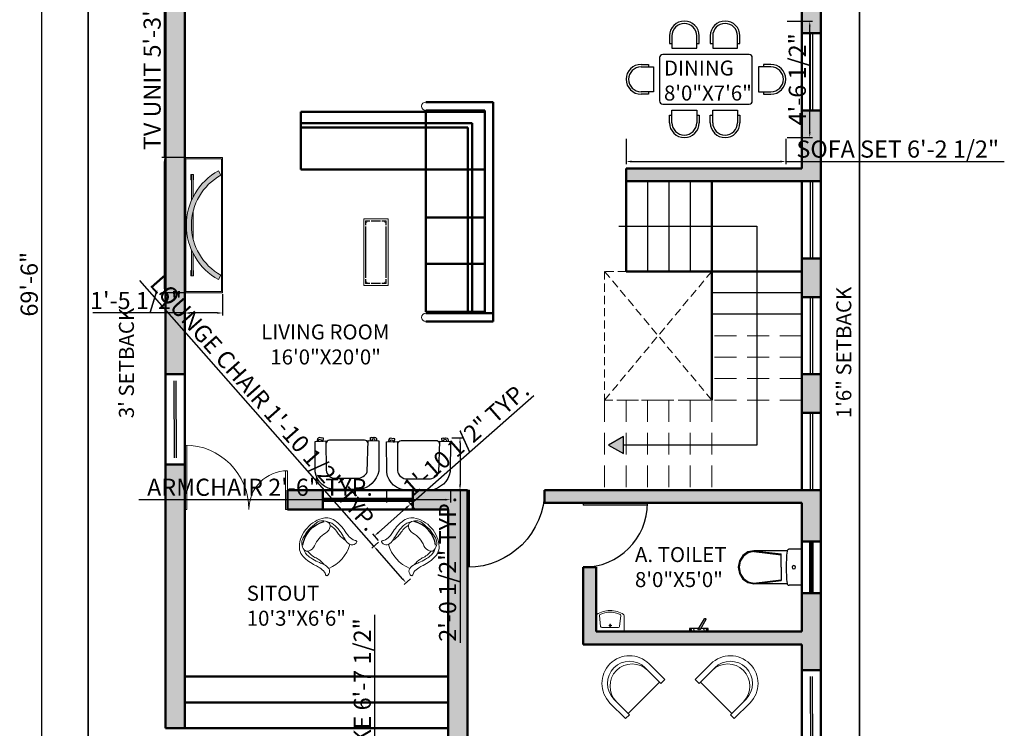
# Model space of a CAD drawing. Units: inches. Extents: x 1986 to 21484, y -1816 to 2016.
# Tile 5 of 85: x 2010 to 2470, y 1277 to 1607. Entities that reach past the tile are written whole.
import ezdxf

# ---------------------------------------------------------------- set-up
doc = ezdxf.new("R2010")
doc.units = ezdxf.units.IN
doc.linetypes.add('DASHED', pattern=[19.05, 12.7, -6.35])
for name, color, linetype in [('2D', 7, 'Continuous'), ('IFF-FURN-DETAIL', 250, 'Continuous'), ('NOI THAT', 42, 'Continuous'), ('SANTEH', 7, 'Continuous')]:
    doc.layers.add(name, color=color, linetype=linetype)
for name, color, linetype, lineweight in [('A-ANNO-DIMS', 2, 'Continuous', 18), ('A-ANNO-TEXT', 7, 'Continuous', 18), ('A-AREA-IDEN', 3, 'Continuous', 18), ('A-DOOR', 3, 'Continuous', 25), ('A-FLOR-FIXT', 8, 'Continuous', 18), ('A-FLOR-STRS', 7, 'Continuous', 25), ('A-FLOR-STRS-OVHD', 8, 'DASHED', 18), ('A-FURN', 8, 'Continuous', 18), ('A-GLAZ', 4, 'Continuous', 25), ('A-WALL', 7, 'Continuous', 50), ('A-WALL-PATT', 8, 'Continuous', 13), ('aparador', 36, 'Continuous', 9), ('C-PROP', 7, 'Continuous', 35), ('moveis', 254, 'Continuous', 5)]:
    doc.layers.add(name, color=color, linetype=linetype, lineweight=lineweight)
doc.styles.get("Standard").update_dxf_attribs({"font": 'arial.ttf'})
doc.dimstyles.new('ISO-25', dxfattribs={"dimtxt": 8, "dimasz": 2.5, "dimexe": 1.25, "dimexo": 0.625, "dimtad": 1, "dimdec": 1, "dimlunit": 3, "dimtxsty": 'Standard', "dimcen": 2.5, "dimadec": 0, "dimazin": 0, "dimtfac": 1, "dimtdec": 1, "dimtmove": 0, "dimatfit": 3, "dimfxl": 1, "dimarcsym": 0})

# ---------------------------------------------------------------- blocks, each defined once
blk = doc.blocks.new('*D2')
at = {"layer": 'A-ANNO-DIMS', "color": 0, "lineweight": -2, "transparency": 16777216}
for p, q in [((2041.69, 1900.75), (2019.21, 1900.75)), ((2020.46, 1898.25), (2020.46, 1069.25)), ((2041.69, 1066.75), (2019.21, 1066.75))]:
    blk.add_line(p, q, dxfattribs=at)
at = {"layer": 'A-ANNO-DIMS', "color": 0, "transparency": 16777216}
for points in [[(2020.05, 1898.25), (2020.88, 1898.25), (2020.46, 1900.75)], [(2020.05, 1069.25), (2020.88, 1069.25), (2020.46, 1066.75)]]:
    blk.add_solid(points, dxfattribs=at)
at = {"layer": 'Defpoints', "color": 0, "transparency": 16777216}
for p in [(2042.31, 1900.75), (2020.46, 1066.75), (2042.31, 1066.75)]:
    blk.add_point(p, dxfattribs=at)
at = {"layer": 'A-ANNO-DIMS', "color": 0, "transparency": 16777216, "insert": (2015.75, 1483.75), "char_height": 8, "attachment_point": 5, "rotation": 90}
blk.add_mtext('69\'-6"', dxfattribs=at)
blk = doc.blocks.new('MD')
for p, q in [((1902.58, 1512.86), (1902.58, 1482.86)), ((1903.58, 1512.86), (1903.58, 1482.86)), ((1949.58, 1482.86), (1949.58, 1500.86)), ((1950.58, 1482.86), (1950.58, 1500.86)), ((1902.58, 1482.86), (1903.58, 1482.86)), ((1949.58, 1482.86), (1950.58, 1482.86))]:
    blk.add_line(p, q)
for centre, radius, start, end in [((1902.58, 1482.86), 30, 0, 90), ((1950.58, 1482.86), 18, 90, 180)]:
    blk.add_arc(centre, radius, start, end)
blk = doc.blocks.new('D2')
for p, q in [((1722.5, 1505.46), (1722.5, 1475.46)), ((1723.5, 1505.46), (1723.5, 1475.46)), ((1722.5, 1475.46), (1723.5, 1475.46))]:
    blk.add_line(p, q)
blk.add_arc((1722.5, 1475.46), 30, 0, 90)
blk = doc.blocks.new('D1')
for p, q in [((1805.96, 1500.36), (1805.96, 1464.36)), ((1806.96, 1500.36), (1806.96, 1464.36)), ((1805.96, 1464.36), (1806.96, 1464.36))]:
    blk.add_line(p, q)
blk.add_arc((1805.96, 1464.36), 36, 0, 90)
blk = doc.blocks.new('WC 2 Symb_109')
at = {"layer": 'SANTEH'}
for p, q in [((0, 0), (0, 380)), ((0, 380), (132, 380)), ((154, 365), (507, 365)), ((506, 365), (216, 331)), ((506, 356), (216, 322)), ((216, 190), (216, 331)), ((216, 190), (216, 49)), ((154, 15), (507, 15)), ((506, 24), (216, 58)), ((506, 15), (216, 49)), ((0, 0), (132, 0))]:
    blk.add_line(p, q, dxfattribs=at)
for points in [[(155, 360), (154, 364), (152, 368), (150, 371), (147, 374), (144, 377), (140, 379), (137, 380), (132, 380)], [(155, 20), (159, 62), (161, 105), (163, 147), (164, 190), (163, 233), (161, 275), (159, 318), (155, 360)], [(506, 24), (565, 37), (616, 73), (649, 126), (661, 190), (649, 254), (616, 307), (565, 343), (506, 356)], [(507, 15), (569, 28), (622, 66), (658, 123), (670, 190), (658, 257), (622, 314), (569, 352), (507, 365)], [(132, 0), (136, 0), (140, 1), (144, 3), (147, 6), (150, 9), (152, 12), (154, 16), (155, 20)]]:
    blk.add_lwpolyline(points, dxfattribs=at)
blk.add_lwpolyline([(84, 208), (70, 203), (65, 190), (70, 177), (84, 172), (97, 177), (102, 190), (97, 203)], close=True, dxfattribs=at)
blk = doc.blocks.new('Faucet - kit sink top')
at = {"layer": 'SANTEH'}
for p, q in [((-5.5, -0.75), (-5.5, -1.25)), ((-4.94278, -0.75), (-5.5, -0.75)), ((-5.5, -1.25), (-4.94278, -1.25)), ((-0.14775, -1.7441), (3.56698, -8.1782)), ((4.43301, -7.6782), (0.71828, -1.2441)), ((4.94278, -0.75), (5.5, -0.75)), ((5.5, -1.25), (4.94278, -1.25)), ((5.5, -0.75), (5.5, -1.25))]:
    blk.add_line(p, q, dxfattribs=at)
blk.add_lwpolyline([(-0.00587, -2), (-6, -2), (-6, 0), (6, 0), (6, -2), (1.15195, -2)], dxfattribs=at)
for centre, radius in [((-4, -1), 1), ((4, -1), 1), ((0, -1), 0.75)]:
    blk.add_circle(centre, radius, dxfattribs=at)
blk.add_arc((4, -7.9282), 0.5, 210, 30, dxfattribs=at)
blk = doc.blocks.new('A$C2EBB240D')
for p, q in [((0, 356), (0, 87)), ((480, 376), (20, 376)), ((500, 356), (500, 87)), ((61, 90), (82, 282)), ((250, 300), (102, 300)), ((250, 300), (398, 300)), ((439, 90), (418, 282))]:
    blk.add_line(p, q)
for points in [[(275, 266), (219, 266)], [(247, 238), (247, 289)]]:
    blk.add_lwpolyline(points)
for centre, radius, start, end in [((20, 356), 20, 90, 180), ((480, 356), 20, 0, 90), ((102, 280), 20, 90, 173.6428), ((247, 266), 16.7, 90, 270), ((247, 266), 10, 90, 270), ((247, 266), 16.7, 270, 90), ((247, 266), 10, 270, 90), ((398, 280), 20, 6.3572, 90), ((20, 87), 20, 180, 237.6892), ((250, 450), 450, 237.6892, 270), ((81, 88), 20, 173.6428, 244.9796), ((250, 450), 420, 244.9796, 270), ((250, 450), 450, 270, 302.3108), ((250, 450), 420, 270, 295.0204), ((419, 88), 20, 295.0204, 6.3572), ((480, 87), 20, 302.3108, 0)]:
    blk.add_arc(centre, radius, start, end)
blk = doc.blocks.new('A$C3F0C2877')
at = {"layer": 'NOI THAT'}
for p, q in [((700, 1640), (700, 1520)), ((740, 1640), (740, 1440)), ((1140, 1440), (1140, 1640)), ((1180, 1520), (1180, 1640)), ((1358, 1640), (1358, 1520)), ((1398, 1640), (1398, 1440)), ((1798, 1440), (1798, 1640)), ((1838, 1520), (1838, 1640)), ((700, 1520), (740, 1520)), ((740, 1440), (1140, 1440)), ((1140, 1520), (1180, 1520)), ((1358, 1520), (1398, 1520)), ((1398, 1440), (1798, 1440)), ((1798, 1520), (1838, 1520)), ((540, 1290), (540, 590)), ((1988, 1340), (590, 1340)), ((2038, 590), (2038, 1290)), ((240, 1180), (360, 1180)), ((240, 1140), (440, 1140)), ((360, 1180), (360, 1140)), ((440, 1140), (440, 740)), ((2139, 1140), (2139, 740)), ((2339, 1140), (2139, 1140)), ((2339, 1180), (2219, 1180)), ((2219, 1180), (2219, 1140)), ((440, 740), (240, 740)), ((360, 700), (240, 700)), ((360, 740), (360, 700)), ((2139, 740), (2339, 740)), ((2219, 740), (2219, 700)), ((2219, 700), (2339, 700)), ((590, 540), (1988, 540)), ((700, 360), (740, 360)), ((700, 240), (700, 360)), ((740, 440), (1140, 440)), ((740, 240), (740, 440)), ((1140, 440), (1140, 240)), ((1140, 360), (1180, 360)), ((1180, 360), (1180, 240)), ((1358, 360), (1398, 360)), ((1358, 240), (1358, 360)), ((1398, 440), (1798, 440)), ((1398, 240), (1398, 440)), ((1798, 440), (1798, 240)), ((1798, 360), (1838, 360)), ((1838, 360), (1838, 240))]:
    blk.add_line(p, q, dxfattribs=at)
for centre, radius, start, end in [((940, 1640), 240, 0, 180), ((940, 1640), 200, 0, 180), ((1598, 1640), 240, 0, 180), ((1598, 1640), 200, 0, 180), ((590, 1290), 50, 90, 180), ((1988, 1290), 50, 0, 90), ((240, 940), 240, 90, 270), ((240, 940), 200, 90, 270), ((2339, 940), 240, 270, 90), ((2339, 940), 200, 270, 90), ((590, 590), 50, 180, 270), ((1988, 590), 50, 270, 0), ((940, 240), 240, 180, 0), ((940, 240), 200, 180, 0), ((1598, 240), 240, 180, 0), ((1598, 240), 200, 180, 0)]:
    blk.add_arc(centre, radius, start, end, dxfattribs=at)
blk = doc.blocks.new('ILNG95')
for points in [[(120, 308, -0.32971), (51, 384, -0.036099), (50, 422, -0.497733), (75, 439, -0.070621), (96, 429, 0.101868), (133, 414, 0.091794), (259, 412, 0.024114), (351, 433, -0.090294), (638, 458, -0.132412), (775, 407, -0.068618), (816, 368, -0.184346), (943, 0, 1.803905)], [(120, 308, 0.138132), (244, 313, 0.001085), (325, 339, -0.034227), (462, 375, -0.033255), (567, 387, -0.137428), (727, 350, -4.561553)], [(120, 308, 0.138132), (244, 313, 0.001085), (325, 339, -0.034227), (462, 375, -0.033255), (567, 387, -0.137428), (727, 350, -4.561553)], [(235, 308, 0.064243), (394, 307, 0.04414), (433, 315, -0.118032), (643, 329, -6.296816)], [(235, 308, 0.064243), (394, 307, 0.04414), (433, 315, -0.118032), (643, 329, -6.296816)], [(639, 0, 0.078302), (612, 161, -0.233633), (633, 315, -0.28763), (710, 349, -0.317923), (875, 193, -0.032882), (900, 0, 1.140397)], [(639, 0, 0.078302), (612, 161, -0.233633), (633, 315, -0.28763), (710, 349, -0.317923), (875, 193, -0.032882), (900, 0, 1.140397)], [(120, -308, 0.32971), (51, -384, 0.036099), (50, -422, 0.497733), (75, -439, 0.070621), (96, -429, -0.101868), (133, -414, -0.091794), (259, -412, -0.024114), (351, -433, 0.090294), (638, -458, 0.132412), (775, -407, 0.068618), (816, -368, 0.184346), (943, 0, -1.803905)], [(639, 0, -0.078302), (612, -161, 0.233633), (633, -315, 0.28763), (710, -349, 0.317923), (875, -193, 0.032882), (900, 0, -1.140397)], [(639, 0, -0.078302), (612, -161, 0.233633), (633, -315, 0.28763), (710, -349, 0.317923), (875, -193, 0.032882), (900, 0, -1.140397)], [(120, -308, -0.138132), (244, -313, -0.001085), (325, -339, 0.034227), (462, -375, 0.033255), (567, -387, 0.137428), (727, -350, 4.561553)], [(120, -308, -0.138132), (244, -313, -0.001085), (325, -339, 0.034227), (462, -375, 0.033255), (567, -387, 0.137428), (727, -350, 4.561553)], [(235, -308, -0.064243), (394, -307, -0.04414), (433, -315, 0.118032), (643, -329, 6.296816)], [(235, -308, -0.064243), (394, -307, -0.04414), (433, -315, 0.118032), (643, -329, 6.296816)]]:
    blk.add_lwpolyline(points, format="xyb")
blk.add_arc((759, 1), 709, 154.3281, 205.801)
at = {"layer": 'IFF-FURN-DETAIL'}
blk.add_arc((326, -2), 549, 326.8997, 34.6691, dxfattribs=at)
blk.add_arc((326, -2), 549, 326.8997, 34.6691, dxfattribs=at)
blk = doc.blocks.new('TABLE-30A')
at = {"color": 0, "linetype": 'ByBlock'}
for p, q in [((0, 0), (0, 0.55)), ((0, 0.55), (1.5, 0.55)), ((0.051, 0.508), (0.042, 0.499)), ((0.042, 0.499), (0.042, 0.478)), ((0.042, 0.478), (0.072, 0.478)), ((0.042, 0.478), (0.042, 0.41)), ((0.072, 0.508), (0.051, 0.508)), ((0.051, 0.478), (0.051, 0.41)), ((0.072, 0.478), (0.072, 0.508)), ((0.072, 0.508), (0.14, 0.508)), ((0.072, 0.499), (0.14, 0.499)), ((1.331, 0.508), (0.169, 0.508)), ((1.331, 0.499), (0.169, 0.499)), ((1.428, 0.508), (1.36, 0.508)), ((1.428, 0.499), (1.36, 0.499)), ((1.428, 0.508), (1.428, 0.478)), ((1.449, 0.508), (1.428, 0.508)), ((1.428, 0.478), (1.458, 0.478)), ((1.458, 0.499), (1.449, 0.508)), ((1.449, 0.478), (1.449, 0.41)), ((1.458, 0.478), (1.458, 0.499)), ((1.458, 0.478), (1.458, 0.41)), ((1.5, 0.55), (1.5, 0)), ((0.042, 0.169), (0.042, 0.381)), ((0.051, 0.169), (0.051, 0.381)), ((1.449, 0.381), (1.449, 0.169)), ((1.458, 0.381), (1.458, 0.169)), ((1.5, 0), (0, 0)), ((0.042, 0.072), (0.042, 0.14)), ((0.042, 0.072), (0.042, 0.051)), ((0.072, 0.072), (0.042, 0.072)), ((0.042, 0.051), (0.051, 0.042)), ((0.051, 0.072), (0.051, 0.14)), ((0.051, 0.042), (0.072, 0.042)), ((0.072, 0.042), (0.072, 0.072)), ((0.072, 0.051), (0.14, 0.051)), ((0.072, 0.042), (0.14, 0.042)), ((0.169, 0.051), (1.331, 0.051)), ((0.169, 0.042), (1.331, 0.042)), ((1.428, 0.051), (1.36, 0.051)), ((1.428, 0.042), (1.36, 0.042)), ((1.428, 0.072), (1.428, 0.042)), ((1.458, 0.072), (1.428, 0.072)), ((1.428, 0.042), (1.449, 0.042)), ((1.449, 0.072), (1.449, 0.14)), ((1.449, 0.042), (1.458, 0.051)), ((1.458, 0.072), (1.458, 0.14)), ((1.458, 0.051), (1.458, 0.072))]:
    blk.add_line(p, q, dxfattribs=at)
blk = doc.blocks.new('S 1')
at = {"layer": '2D'}
blk.add_lwpolyline([(4300.17, 1811.07), (4294.36, 1811.27), (4294.5, 1827.76, -0.326306), (4305.18, 1837.77), (4318.07, 1837.77, -0.372891), (4329.09, 1828.23), (4329.16, 1811.54), (4323.28, 1811.34), (4323.21, 1827.16, 0.399039), (4317.87, 1831.63), (4306.12, 1831.63, 0.288471), (4300.71, 1828.23)], format="xyb", close=True, dxfattribs=at)
for points in [[(4296.37, 1811.14), (4296.63, 1810.34), (4297.23, 1810.21), (4298.1, 1810.54), (4298.1, 1811.14), (4298.9, 1811.14), (4299.04, 1809.54), (4298.24, 1809.34), (4298.17, 1809.61), (4296.9, 1809.27), (4296.17, 1809.47), (4295.77, 1809.94), (4295.63, 1810.74), (4295.63, 1811.21)], [(4327.35, 1811.41), (4327.09, 1810.61), (4326.49, 1810.47), (4325.62, 1810.81), (4325.62, 1811.41), (4324.82, 1811.41), (4324.68, 1809.81), (4325.48, 1809.61), (4325.55, 1809.87), (4326.82, 1809.54), (4327.55, 1809.74), (4327.95, 1810.21), (4328.09, 1811.01), (4328.09, 1811.47)]]:
    blk.add_lwpolyline(points, dxfattribs=at)
blk.add_lwpolyline([(4300.24, 1812.34, 0.33845), (4302.18, 1810.94), (4321.28, 1810.94, 0.381322), (4323.15, 1812.61, -0.892406)], format="xyb", dxfattribs=at)
blk = doc.blocks.new('12PSTG07')
at = {"color": 0, "linetype": 'ByBlock'}
for p, q in [((0, 15), (-12, 15)), ((-12, 12), (0, 12)), ((-1, -12), (-1, 12)), ((0, 12), (0, 15)), ((-12, -12), (0, -12)), ((0, -15), (-12, -15)), ((0, -12), (0, -15))]:
    blk.add_line(p, q, dxfattribs=at)
for centre, radius in [((-12, 0), 15), ((-12, 0), 12), ((-10, 0), 12)]:
    blk.add_arc(centre, radius, 90, 270, dxfattribs=at)
blk = doc.blocks.new('Aparador ORGANICA Formatto')
at = {"layer": 'aparador', "ltscale": 0.3}
h = blk.add_hatch(color=256, dxfattribs=at)
h.dxf.hatch_style = 1
h.set_gradient(color1=(118, 213, 123), color2=(52, 168, 57), one_color=1, tint=0.43, name='INVCURVED')
h.paths.add_polyline_path([(0.8, 0.45), (-0.8, 0.45), (-0.8, 0), (0.8, 0)])
h.paths.add_polyline_path([(0.785, 0.435), (0.785, 0.015), (-0.785, 0.015), (-0.785, 0.435)], flags=16)
h.paths.add_polyline_path([(0.291, 0.37), (0.537, 0.37), (0.537, 0.376), (0.601, 0.376), (0.601, 0.37), (0.601, 0.35), (0.601, 0.344), (0.537, 0.344), (0.537, 0.35), (0.334, 0.35, -0.150336), (0.645, 0.049), (0.592, 0.02, 0.208852), (0.163, 0.35), (-0.163, 0.35, 0.208852), (-0.592, 0.02), (-0.645, 0.049, -0.150336), (-0.334, 0.35), (-0.537, 0.35), (-0.537, 0.344), (-0.601, 0.344), (-0.601, 0.35), (-0.601, 0.37), (-0.601, 0.376), (-0.537, 0.376), (-0.537, 0.37), (-0.291, 0.37, -0.206106)], flags=0)
h = blk.add_hatch(color=256, dxfattribs=at)
h.dxf.hatch_style = 1
h.set_gradient(color1=(135, 92, 69), color2=(0, 0, 0), one_color=1, name='INVCURVED')
h.paths.add_polyline_path([(-0.645, 0.049), (-0.592, 0.02, -0.590888), (0.592, 0.02), (0.645, 0.049, 0.590888)])
h = blk.add_hatch(color=256, dxfattribs=at)
h.dxf.hatch_style = 1
h.set_gradient(color1=(178, 189, 189), one_color=1, tint=1, name='CYLINDER')
h.paths.add_polyline_path([(-0.537, 0.376), (-0.601, 0.376), (-0.601, 0.37), (-0.537, 0.37)])
h.paths.add_polyline_path([(-0.537, 0.35), (-0.601, 0.35), (-0.601, 0.344), (-0.537, 0.344)])
h = blk.add_hatch(color=256, dxfattribs=at)
h.dxf.hatch_style = 1
h.set_gradient(color1=(118, 213, 123), color2=(31, 101, 35), one_color=1, tint=0.26, name='INVCURVED')
h.paths.add_polyline_path([(-0.291, 0.37), (-0.601, 0.37), (-0.601, 0.35), (-0.334, 0.35, -0.015999)])
h = blk.add_hatch(color=256, dxfattribs=at)
h.dxf.hatch_style = 1
h.set_gradient(color1=(118, 213, 123), color2=(31, 101, 35), one_color=1, tint=0.26, name='INVCURVED')
h.paths.add_polyline_path([(-0.163, 0.35), (0.163, 0.35, 0.122516)])
h = blk.add_hatch(color=256, dxfattribs=at)
h.dxf.hatch_style = 1
h.set_gradient(color1=(118, 213, 123), color2=(31, 101, 35), one_color=1, tint=0.26, name='INVCURVED')
h.paths.add_polyline_path([(0.601, 0.37), (0.291, 0.37, -0.015999), (0.334, 0.35), (0.601, 0.35)])
h = blk.add_hatch(color=256, dxfattribs=at)
h.dxf.hatch_style = 1
h.set_gradient(color1=(178, 189, 189), one_color=1, tint=1, name='CYLINDER')
h.paths.add_polyline_path([(0.601, 0.376), (0.537, 0.376), (0.537, 0.37), (0.601, 0.37)])
h.paths.add_polyline_path([(0.601, 0.35), (0.537, 0.35), (0.537, 0.344), (0.601, 0.344)])
for p, q in [((-0.592, 0.02), (-0.645, 0.049)), ((0.592, 0.02), (0.645, 0.049))]:
    blk.add_line(p, q, dxfattribs=at)
for points in [[(-0.601, 0.37), (-0.601, 0.376), (-0.537, 0.376), (-0.537, 0.37)], [(0.601, 0.37), (0.601, 0.376), (0.537, 0.376), (0.537, 0.37)], [(-0.537, 0.35), (-0.537, 0.344), (-0.601, 0.344), (-0.601, 0.35)], [(0.537, 0.35), (0.537, 0.344), (0.601, 0.344), (0.601, 0.35)]]:
    blk.add_lwpolyline(points, dxfattribs=at)
for radius in [0.736, 0.676]:
    blk.add_arc((0, -0.306), radius, 28.8434, 151.1566, dxfattribs=at)
at = {"layer": 'moveis', "ltscale": 0.3}
for p, q in [((-0.601, 0.37), (-0.601, 0.35)), ((-0.291, 0.37), (-0.601, 0.37)), ((0.291, 0.37), (0.601, 0.37)), ((0.601, 0.37), (0.601, 0.35)), ((-0.601, 0.35), (-0.334, 0.35)), ((-0.163, 0.35), (0.163, 0.35)), ((0.601, 0.35), (0.334, 0.35))]:
    blk.add_line(p, q, dxfattribs=at)
for points in [[(-0.8, 0), (0.8, 0), (0.8, 0.45), (-0.8, 0.45)], [(-0.785, 0.015), (0.785, 0.015), (0.785, 0.435), (-0.785, 0.435)]]:
    blk.add_lwpolyline(points, close=True, dxfattribs=at)
blk = doc.blocks.new('WIN-36')
for p, q in [((0, 36), (0, 0)), ((0, 36), (0, 0)), ((1, 36), (1, 0))]:
    blk.add_line(p, q)
blk = doc.blocks.new('*D105')
at = {"layer": 'A-ANNO-DIMS', "color": 0, "lineweight": -2, "transparency": 16777216}
for p, q in [((2175.61, 1361.57), (2066.34, 1485.46)), ((2177.71, 1363.41), (2174.68, 1360.74)), ((2189.01, 1346.38), (2177.27, 1359.69)), ((2192.75, 1346.35), (2189.72, 1343.68))]:
    blk.add_line(p, q, dxfattribs=at)
at = {"layer": 'A-ANNO-DIMS', "color": 0, "transparency": 16777216}
for points in [[(2177.58, 1359.97), (2176.96, 1359.42), (2175.61, 1361.57)], [(2189.32, 1346.66), (2188.7, 1346.11), (2190.66, 1344.51)]]:
    blk.add_solid(points, dxfattribs=at)
at = {"layer": 'Defpoints', "color": 0, "transparency": 16777216}
for p in [(2175.61, 1361.57), (2178.17, 1363.82), (2193.22, 1346.76)]:
    blk.add_point(p, dxfattribs=at)
at = {"layer": 'A-ANNO-DIMS', "color": 0, "transparency": 16777216, "insert": (2123.73, 1427.6), "char_height": 8, "attachment_point": 5, "rotation": 311.4119}
blk.add_mtext('LOUNGE CHAIR 1\'-10 1/2" TYP.', dxfattribs=at)
blk = doc.blocks.new('*D106')
at = {"layer": 'A-ANNO-DIMS', "color": 0, "lineweight": -2, "transparency": 16777216}
for p, q in [((2192.75, 1381.23), (2250.21, 1431.91)), ((2177.79, 1368.04), (2190.87, 1379.58)), ((2194.59, 1379.14), (2191.92, 1382.17)), ((2177.76, 1364.29), (2175.09, 1367.32))]:
    blk.add_line(p, q, dxfattribs=at)
at = {"layer": 'A-ANNO-DIMS', "color": 0, "transparency": 16777216}
for points in [[(2190.6, 1379.89), (2191.15, 1379.26), (2192.75, 1381.23)], [(2177.52, 1368.35), (2178.07, 1367.72), (2175.92, 1366.38)]]:
    blk.add_solid(points, dxfattribs=at)
at = {"layer": 'Defpoints', "color": 0, "transparency": 16777216}
for p in [(2192.75, 1381.23), (2195.01, 1378.67), (2178.17, 1363.82)]:
    blk.add_point(p, dxfattribs=at)
at = {"layer": 'A-ANNO-DIMS', "color": 0, "transparency": 16777216, "insert": (2219.27, 1410.97), "char_height": 8, "attachment_point": 5, "rotation": 41.4119}
blk.add_mtext('1\'-10 1/2" TYP.', dxfattribs=at)
blk = doc.blocks.new('*D107')
at = {"layer": 'A-ANNO-DIMS', "color": 0, "lineweight": -2, "transparency": 16777216}
for p, q in [((2181.56, 1387.13), (2181.56, 1382.03)), ((2211.35, 1387.13), (2211.35, 1382.03)), ((2181.56, 1383.28), (2065.87, 1383.28)), ((2208.85, 1383.28), (2184.06, 1383.28))]:
    blk.add_line(p, q, dxfattribs=at)
at = {"layer": 'A-ANNO-DIMS', "color": 0, "transparency": 16777216}
for points in [[(2184.06, 1383.7), (2184.06, 1382.87), (2181.56, 1383.28)], [(2208.85, 1383.7), (2208.85, 1382.87), (2211.35, 1383.28)]]:
    blk.add_solid(points, dxfattribs=at)
at = {"layer": 'Defpoints', "color": 0, "transparency": 16777216}
for p in [(2181.56, 1387.75), (2211.35, 1387.75), (2181.56, 1383.28)]:
    blk.add_point(p, dxfattribs=at)
at = {"layer": 'A-ANNO-DIMS', "color": 0, "transparency": 16777216, "insert": (2122.46, 1388.04), "char_height": 8, "attachment_point": 5}
blk.add_mtext('ARMCHAIR 2\'-6" TYP.', dxfattribs=at)
blk = doc.blocks.new('*D108')
at = {"layer": 'A-ANNO-DIMS', "color": 0, "lineweight": -2, "transparency": 16777216}
for p, q in [((2211.98, 1412.16), (2217.07, 1412.16)), ((2215.82, 1409.66), (2215.82, 1390.25)), ((2211.98, 1387.75), (2217.07, 1387.75)), ((2215.82, 1387.75), (2215.82, 1316.46))]:
    blk.add_line(p, q, dxfattribs=at)
at = {"layer": 'A-ANNO-DIMS', "color": 0, "transparency": 16777216}
for points in [[(2215.41, 1409.66), (2216.24, 1409.66), (2215.82, 1412.16)], [(2215.41, 1390.25), (2216.24, 1390.25), (2215.82, 1387.75)]]:
    blk.add_solid(points, dxfattribs=at)
at = {"layer": 'Defpoints', "color": 0, "transparency": 16777216}
for p in [(2211.35, 1412.16), (2211.35, 1387.75), (2215.82, 1387.75)]:
    blk.add_point(p, dxfattribs=at)
at = {"layer": 'A-ANNO-DIMS', "color": 0, "transparency": 16777216, "insert": (2211.06, 1350.86), "char_height": 8, "attachment_point": 5, "rotation": 90}
blk.add_mtext('2\'-0 1/2" TYP.', dxfattribs=at)
blk = doc.blocks.new('*D115')
at = {"layer": 'A-ANNO-DIMS', "color": 0, "lineweight": -2, "transparency": 16777216}
for p, q in [((2293.37, 1551.52), (2293.37, 1539.72)), ((2367.88, 1551.52), (2367.88, 1539.72)), ((2295.87, 1540.97), (2365.38, 1540.97)), ((2367.88, 1540.97), (2469.87, 1540.97))]:
    blk.add_line(p, q, dxfattribs=at)
at = {"layer": 'A-ANNO-DIMS', "color": 0, "transparency": 16777216}
for points in [[(2295.87, 1541.39), (2295.87, 1540.56), (2293.37, 1540.97)], [(2365.38, 1541.39), (2365.38, 1540.56), (2367.88, 1540.97)]]:
    blk.add_solid(points, dxfattribs=at)
at = {"layer": 'Defpoints', "color": 0, "transparency": 16777216}
for p in [(2293.37, 1552.15), (2367.88, 1552.15), (2367.88, 1540.97)]:
    blk.add_point(p, dxfattribs=at)
at = {"layer": 'A-ANNO-DIMS', "color": 0, "transparency": 16777216, "insert": (2420.13, 1545.74), "char_height": 8, "attachment_point": 5}
blk.add_mtext('SOFA SET 6\'-2 1/2"', dxfattribs=at)
blk = doc.blocks.new('*D116')
at = {"layer": 'A-ANNO-DIMS', "color": 0, "lineweight": -2, "transparency": 16777216}
for p, q in [((2368.5, 1606.47), (2380.31, 1606.47)), ((2379.06, 1554.65), (2379.06, 1603.97)), ((2368.5, 1552.15), (2380.31, 1552.15))]:
    blk.add_line(p, q, dxfattribs=at)
at = {"layer": 'A-ANNO-DIMS', "color": 0, "transparency": 16777216}
for points in [[(2378.64, 1603.97), (2379.47, 1603.97), (2379.06, 1606.47)], [(2378.64, 1554.65), (2379.47, 1554.65), (2379.06, 1552.15)]]:
    blk.add_solid(points, dxfattribs=at)
at = {"layer": 'Defpoints', "color": 0, "transparency": 16777216}
for p in [(2367.88, 1606.47), (2379.06, 1606.47), (2367.88, 1552.15)]:
    blk.add_point(p, dxfattribs=at)
at = {"layer": 'A-ANNO-DIMS', "color": 0, "transparency": 16777216, "insert": (2374.29, 1579.31), "char_height": 8, "attachment_point": 5, "rotation": 90}
blk.add_mtext('4\'-6 1/2"', dxfattribs=at)
blk = doc.blocks.new('*D119')
at = {"layer": 'A-ANNO-DIMS', "color": 0, "lineweight": -2, "transparency": 16777216}
for p, q in [((2077.86, 1542.78), (2077.86, 1614.56)), ((2086.69, 1542.78), (2076.61, 1542.78)), ((2077.86, 1482.29), (2077.86, 1540.28)), ((2086.69, 1479.79), (2076.61, 1479.79))]:
    blk.add_line(p, q, dxfattribs=at)
at = {"layer": 'A-ANNO-DIMS', "color": 0, "transparency": 16777216}
for points in [[(2077.45, 1540.28), (2078.28, 1540.28), (2077.86, 1542.78)], [(2077.45, 1482.29), (2078.28, 1482.29), (2077.86, 1479.79)]]:
    blk.add_solid(points, dxfattribs=at)
at = {"layer": 'Defpoints', "color": 0, "transparency": 16777216}
for p in [(2077.86, 1542.78), (2087.31, 1542.78), (2087.31, 1479.79)]:
    blk.add_point(p, dxfattribs=at)
at = {"layer": 'A-ANNO-DIMS', "color": 0, "transparency": 16777216, "insert": (2073.15, 1579.92), "char_height": 8, "attachment_point": 5, "rotation": 90}
blk.add_mtext('TV UNIT 5\'-3"', dxfattribs=at)
blk = doc.blocks.new('*D120')
at = {"layer": 'A-ANNO-DIMS', "color": 0, "lineweight": -2, "transparency": 16777216}
for p, q in [((2087.31, 1479.16), (2087.31, 1469.09)), ((2105.03, 1479.16), (2105.03, 1469.09)), ((2087.31, 1470.34), (2044.41, 1470.34)), ((2102.53, 1470.34), (2089.81, 1470.34))]:
    blk.add_line(p, q, dxfattribs=at)
at = {"layer": 'A-ANNO-DIMS', "color": 0, "transparency": 16777216}
for points in [[(2089.81, 1470.76), (2089.81, 1469.92), (2087.31, 1470.34)], [(2102.53, 1470.76), (2102.53, 1469.92), (2105.03, 1470.34)]]:
    blk.add_solid(points, dxfattribs=at)
at = {"layer": 'Defpoints', "color": 0, "transparency": 16777216}
for p in [(2087.31, 1479.79), (2105.03, 1479.79), (2087.31, 1470.34)]:
    blk.add_point(p, dxfattribs=at)
at = {"layer": 'A-ANNO-DIMS', "color": 0, "transparency": 16777216, "insert": (2064.61, 1475.1), "char_height": 8, "attachment_point": 5}
blk.add_mtext('1\'-5 1/2"', dxfattribs=at)
blk = doc.blocks.new('*D125')
at = {"layer": 'A-ANNO-DIMS', "color": 0, "lineweight": -2, "transparency": 16777216}
for p, q in [((2176.01, 1216.11), (2176.01, 1329.57)), ((2164.68, 1216.11), (2177.26, 1216.11)), ((2176.01, 1138.94), (2176.01, 1213.61)), ((2164.68, 1136.44), (2177.26, 1136.44))]:
    blk.add_line(p, q, dxfattribs=at)
at = {"layer": 'A-ANNO-DIMS', "color": 0, "transparency": 16777216}
for points in [[(2175.59, 1213.61), (2176.42, 1213.61), (2176.01, 1216.11)], [(2175.59, 1138.94), (2176.42, 1138.94), (2176.01, 1136.44)]]:
    blk.add_solid(points, dxfattribs=at)
at = {"layer": 'Defpoints', "color": 0, "transparency": 16777216}
for p in [(2164.06, 1216.11), (2176.01, 1216.11), (2164.06, 1136.44)]:
    blk.add_point(p, dxfattribs=at)
at = {"layer": 'A-ANNO-DIMS', "color": 0, "transparency": 16777216, "insert": (2171.24, 1274.09), "char_height": 8, "attachment_point": 5, "rotation": 90}
blk.add_mtext('MOTORBIKE 6\'-7 1/2"', dxfattribs=at)

msp = doc.modelspace()

# ---------------------------------------------------------------- hatches: boundary and pattern name
at = {"layer": 'A-FLOR-STRS'}
h = msp.add_hatch(color=256, dxfattribs=at)
h.dxf.hatch_style = 1
h.paths.add_polyline_path([(2285.15, 1408.75), (2292.11, 1404.74), (2292.11, 1412.77)])
at = {"layer": 'A-WALL-PATT'}
h = msp.add_hatch(color=256, dxfattribs=at)
h.dxf.hatch_style = 1
h.paths.add_polyline_path([(2087.31, 1843.75), (2135.31, 1843.75), (2135.31, 1852.75), (2078.31, 1852.75), (2078.31, 1753.75), (2087.31, 1753.75)])
h.paths.add_polyline_path([(2231.31, 1852.75), (2177.31, 1852.75), (2177.31, 1843.75), (2225.31, 1843.75), (2225.31, 1627.75), (2231.31, 1627.75), (2231.31, 1633.35), (2231.31, 1676.45), (2231.31, 1678.13)])
h.paths.add_polyline_path([(2384.31, 1852.75), (2261.31, 1852.75), (2261.31, 1843.75), (2375.31, 1843.75), (2375.31, 1795.75), (2279.31, 1795.75), (2279.31, 1813.75), (2273.31, 1813.75), (2273.31, 1789.75), (2375.31, 1789.75), (2375.31, 1741.75), (2384.31, 1741.75)])
h.paths.add_polyline_path([(2384.31, 1705.75), (2375.31, 1705.75), (2375.31, 1600.75), (2384.31, 1600.75)])
h.paths.add_polyline_path([(2384.31, 1564.75), (2375.31, 1564.75), (2375.31, 1537.75), (2293.31, 1537.75), (2293.31, 1531.75), (2375.31, 1531.75), (2384.31, 1531.75)])
h.paths.add_polyline_path([(2087.31, 1711.75), (2078.31, 1711.75), (2078.31, 1669.75), (2087.31, 1669.75), (2087.31, 1681.75), (2177.31, 1681.75), (2177.31, 1663.75), (2183.31, 1663.75), (2183.31, 1681.75), (2189.31, 1681.75), (2189.31, 1687.75), (2087.31, 1687.75)])
h.paths.add_polyline_path([(2087.31, 1627.75), (2183.31, 1627.75), (2183.31, 1633.75), (2153.31, 1633.75), (2087.31, 1633.75), (2087.31, 1645.75), (2078.31, 1645.75), (2078.31, 1441.75), (2087.31, 1441.75)])
h.paths.add_polyline_path([(2087.31, 1399.75), (2078.31, 1399.75), (2078.31, 1276.75), (2087.31, 1276.75)])
h.paths.add_polyline_path([(2151.81, 1387.75), (2135.31, 1387.75), (2135.31, 1378.75), (2151.81, 1378.75)])
h.paths.add_polyline_path([(2219.31, 1387.75), (2193.81, 1387.75), (2193.81, 1378.75), (2210.31, 1378.75), (2210.31, 1189.75), (2219.31, 1189.75)])
h.paths.add_polyline_path([(2384.31, 1387.75), (2375.31, 1387.75), (2255.31, 1387.75), (2255.31, 1381.75), (2375.31, 1381.75), (2375.31, 1363.75), (2384.31, 1363.75)])
h.paths.add_polyline_path([(2384.31, 1339.75), (2375.31, 1339.75), (2375.31, 1321.75), (2279.31, 1321.75), (2279.31, 1351.75), (2273.31, 1351.75), (2273.31, 1315.75), (2375.31, 1315.75), (2375.31, 1303.75), (2384.31, 1303.75)])
h.paths.add_polyline_path([(2225.31, 1123.75), (2219.31, 1123.75), (2219.31, 1147.75), (2210.31, 1147.75), (2210.31, 1114.75), (2225.31, 1114.75)])
h.paths.add_polyline_path([(2384.31, 1147.75), (2375.31, 1147.75), (2375.31, 1123.75), (2267.31, 1123.75), (2267.31, 1114.75), (2384.31, 1114.75)])
h.paths.add_polyline_path([(2384.31, 1261.75), (2375.31, 1261.75), (2375.31, 1189.75), (2384.31, 1189.75)])
h.paths.add_polyline_path([(2384.31, 1441.75), (2375.31, 1441.75), (2375.31, 1423.75), (2384.31, 1423.75)])
h.paths.add_polyline_path([(2384.31, 1495.75), (2375.31, 1495.75), (2375.31, 1477.75), (2384.31, 1477.75)])

# ---------------------------------------------------------------- linework, layer by layer
at = {"layer": 'A-FLOR-STRS'}
for p, q in [((2303.31, 1531.75), (2303.31, 1489.75)), ((2313.31, 1531.75), (2313.31, 1489.75)), ((2323.31, 1531.75), (2323.31, 1489.75)), ((2375.31, 1479.75), (2333.31, 1479.75)), ((2375.31, 1469.75), (2333.31, 1469.75))]:
    msp.add_line(p, q, dxfattribs=at)
msp.add_lwpolyline([(2289.9, 1510.75), (2354.31, 1510.75), (2354.31, 1408.75), (2292.11, 1408.75)], dxfattribs=at)
msp.add_lwpolyline([(2285.15, 1408.75), (2292.11, 1404.74), (2292.11, 1412.77)], close=True, dxfattribs=at)
at = {"layer": 'A-FLOR-STRS-OVHD', "ltscale": 0.3}
for p, q in [((2283.31, 1489.75), (2333.31, 1429.75)), ((2283.31, 1429.75), (2333.31, 1489.75))]:
    msp.add_line(p, q, dxfattribs=at)
at = {"layer": 'A-FLOR-STRS-OVHD', "ltscale": 0.8}
for p, q in [((2375.31, 1459.75), (2333.31, 1459.75)), ((2375.31, 1449.75), (2333.31, 1449.75)), ((2375.31, 1439.75), (2333.31, 1439.75)), ((2375.31, 1429.75), (2283.31, 1429.75)), ((2283.31, 1429.75), (2283.31, 1387.75)), ((2293.31, 1429.75), (2293.31, 1387.75)), ((2303.31, 1429.75), (2303.31, 1387.75)), ((2313.31, 1429.75), (2313.31, 1387.75)), ((2323.31, 1429.75), (2323.31, 1387.75)), ((2333.31, 1429.75), (2333.31, 1387.75))]:
    msp.add_line(p, q, dxfattribs=at)
at = {"layer": 'A-FLOR-STRS-OVHD', "ltscale": 0.3}
msp.add_lwpolyline([(2283.31, 1429.75), (2333.31, 1429.75), (2333.31, 1489.75), (2283.31, 1489.75)], close=True, dxfattribs=at)
at = {"layer": 'A-FURN'}
for centre in [(2199.82, 1566.73), (2199.82, 1468.31)]:
    msp.add_arc(centre, 1.97, 90, 270, dxfattribs=at)
at = {"layer": 'A-WALL'}
for p, q in [((2384.31, 1900.75), (2384.31, 1114.75)), ((2078.31, 1276.75), (2078.31, 1852.75)), ((2375.31, 1789.75), (2375.31, 1537.75)), ((2087.31, 1276.75), (2087.31, 1627.75)), ((2375.31, 1600.75), (2384.31, 1600.75)), ((2199.82, 1568.7), (2231.31, 1568.7)), ((2231.31, 1568.7), (2231.31, 1466.34)), ((2141.59, 1564.11), (2141.59, 1537.21)), ((2227.38, 1564.11), (2141.59, 1564.11)), ((2199.82, 1564.76), (2227.38, 1564.76)), ((2199.82, 1470.93), (2199.82, 1564.11)), ((2227.38, 1564.76), (2227.38, 1470.93)), ((2375.31, 1564.75), (2384.31, 1564.75)), ((2141.59, 1558.86), (2221.47, 1558.86)), ((2221.47, 1558.86), (2221.47, 1470.93)), ((2141.59, 1556.89), (2219.5, 1556.89)), ((2219.5, 1556.89), (2219.5, 1470.93)), ((2227.38, 1537.21), (2141.59, 1537.21)), ((2205.06, 1537.21), (2141.59, 1537.21)), ((2293.31, 1537.75), (2375.31, 1537.75)), ((2293.31, 1537.75), (2293.31, 1489.75)), ((2293.31, 1531.75), (2375.31, 1531.75)), ((2333.31, 1531.75), (2333.31, 1429.75)), ((2375.31, 1531.75), (2375.31, 1387.75)), ((2375.31, 1531.75), (2384.31, 1531.75)), ((2227.38, 1514.89), (2199.82, 1514.89)), ((2375.31, 1495.75), (2384.31, 1495.75)), ((2227.38, 1493.24), (2199.82, 1493.24)), ((2375.31, 1489.75), (2293.31, 1489.75)), ((2375.31, 1477.75), (2384.31, 1477.75)), ((2227.38, 1470.93), (2199.82, 1470.93)), ((2231.31, 1470.27), (2199.82, 1470.27)), ((2231.31, 1466.34), (2199.82, 1466.34)), ((2078.31, 1441.75), (2087.31, 1441.75)), ((2375.31, 1441.75), (2384.31, 1441.75)), ((2375.31, 1423.75), (2384.31, 1423.75)), ((2078.31, 1399.75), (2087.31, 1399.75)), ((2135.31, 1387.75), (2219.31, 1387.75)), ((2135.31, 1378.75), (2135.31, 1387.75)), ((2151.81, 1378.75), (2151.81, 1387.75)), ((2151.81, 1383.75), (2193.81, 1383.75)), ((2193.81, 1378.75), (2193.81, 1387.75)), ((2219.31, 1123.75), (2219.31, 1387.75)), ((2255.31, 1381.75), (2255.31, 1387.75)), ((2255.31, 1387.75), (2375.31, 1387.75)), ((2375.31, 1387.75), (2384.31, 1387.75)), ((2135.31, 1378.75), (2210.31, 1378.75)), ((2151.81, 1382.75), (2193.81, 1382.75)), ((2210.31, 1114.75), (2210.31, 1378.75)), ((2255.31, 1381.75), (2375.31, 1381.75)), ((2375.31, 1381.75), (2375.31, 1321.75)), ((2375.31, 1363.75), (2384.31, 1363.75)), ((2379.31, 1339.75), (2379.31, 1363.75)), ((2380.31, 1339.75), (2380.31, 1363.75)), ((2273.31, 1351.75), (2273.31, 1315.75)), ((2273.31, 1351.75), (2279.31, 1351.75)), ((2279.31, 1351.75), (2279.31, 1321.75)), ((2375.31, 1339.75), (2384.31, 1339.75)), ((2279.31, 1321.75), (2375.31, 1321.75)), ((2273.31, 1315.75), (2375.31, 1315.75)), ((2375.31, 1315.75), (2375.31, 1123.75)), ((2087.31, 1300.75), (2210.31, 1300.75)), ((2375.31, 1303.75), (2384.31, 1303.75)), ((2087.31, 1288.75), (2210.31, 1288.75)), ((2078.31, 1276.75), (2210.31, 1276.75))]:
    msp.add_line(p, q, dxfattribs=at)
at = {"layer": 'C-PROP'}
msp.add_lwpolyline([(2042.31, 1900.75), (2402.31, 1900.75), (2402.31, 1066.75), (2042.31, 1066.75)], close=True, dxfattribs=at)

# ---------------------------------------------------------------- block references
at = {"layer": 'A-DOOR', "xscale": -1, "rotation": 180}
msp.add_blockref('D1', (413.35, 2852.11), dxfattribs=at)
at = {"layer": 'A-DOOR', "rotation": 270}
msp.add_blockref('D2', (797.86, 3104.25), dxfattribs=at)
at = {"layer": 'A-FLOR-FIXT'}
for name, p, xscale, yscale, zscale, rotation in [('WC 2 Symb_109', (2375.31, 1360.15), 0.0441898926459964, 0.0441898926459964, 0.0441898926459964, 180), ('A$C2EBB240D', (2292.42, 1331.6), 0.026211548048557, 0.026211548048557, 0.026211548048557, 180), ('Faucet - kit sink top', (2327.31, 1321.75), -0.7356136897818673, 0.7356136897818673, 0.7356136897818673, 180), ('12PSTG07', (2302.23, 1290.29), 0.8597921787217943, 0.8597921787217943, 0.8597921787217943, 315), ('12PSTG07', (2334.74, 1290.29), -0.8597921787217945, 0.8597921787217943, 0.8597921787217943, 45)]:
    msp.add_blockref(name, p, dxfattribs=dict(at, xscale=xscale, yscale=yscale, zscale=zscale, rotation=rotation))
at = {"layer": 'A-FURN', "xscale": 0.0288952394299788, "yscale": 0.0288952394299788, "zscale": 0.0288952394299788}
msp.add_blockref('A$C3F0C2877', (2293.37, 1552.15), dxfattribs=at)
at = {"layer": 'A-FURN'}
for name, p, xscale, yscale, zscale, rotation in [('Aparador ORGANICA Formatto', (2105.03, 1511.28), 39.3701, 39.3701, 39.3701, 90), ('TABLE-30A', (2170.88, 1514.24), 20.70834898381633, 20.70834898381633, 20.70834898381633, 270), ('S 1', (5855.3, 2961.73), 0.8563117011609614, 0.8563117011609614, 0.8563117011609614, 180), ('S 1', (5888.67, 2961.46), 0.8563117011609614, 0.8563117011609614, 0.8563117011609614, 180), ('ILNG95', (2161.69, 1354.87), -0.0243705291132055, 0.0243705291132055, 0.0243705291132055, 318.5881218623716), ('ILNG95', (2185.21, 1354.87), 0.0243705291132055, 0.0243705291132055, 0.0243705291132055, 41.41187813762839)]:
    msp.add_blockref(name, p, dxfattribs=dict(at, xscale=xscale, yscale=yscale, zscale=zscale, rotation=rotation))
msp.add_blockref('MD', (184.73, -104.11), dxfattribs=at)
at = {"layer": 'A-GLAZ'}
for p in [(2379.31, 1564.75), (2379.31, 1495.75), (2379.31, 1441.75), (2379.31, 1387.75)]:
    msp.add_blockref('WIN-36', p, dxfattribs=at)
at = {"layer": 'A-GLAZ', "rotation": 0.302793432207276}
for p in [(2082.41, 1402.75), (2379.41, 1264.75)]:
    msp.add_blockref('WIN-36', p, dxfattribs=at)

# ---------------------------------------------------------------- texts
at = {"layer": 'A-ANNO-TEXT', "char_height": 7, "attachment_point": 1, "rotation": 90}
for s, insert in [('{\\fTimes New Roman|b0|i0|c0|p18;1\'6" SETBACK}', (2391.45, 1421.26)), ("{\\fTimes New Roman|b0|i0|c0|p18;3' SETBACK}", (2056.62, 1421.26))]:
    msp.add_mtext_dynamic_manual_height_columns(s, width=105.6127, gutter_width=12.5, heights=[0], dxfattribs=dict(at, insert=insert))
at = {"layer": 'A-AREA-IDEN', "char_height": 7, "attachment_point": 1}
for s, width, insert in [('{\\fTimes New Roman|b0|i0|c0|p18;DINING\\P8\'0"X7\'6"}', 105.6127, (2311.01, 1588.07)), ('{\\fTimes New Roman|b0|i0|c0|p18;LIVING ROOM\\P  16\'0"X20\'0"}', 122.2228, (2122.99, 1465)), ('{\\fTimes New Roman|b0|i0|c0|p18;A. TOILET\\P8\'0"X5\'0"}', 105.6127, (2297.48, 1361.19)), ('{\\fTimes New Roman|b0|i0|c0|p18;SITOUT\\P10\'3"X6\'6"}', 105.6127, (2116.26, 1343.16))]:
    msp.add_mtext_dynamic_manual_height_columns(s, width=width, gutter_width=12.5, heights=[0], dxfattribs=dict(at, insert=insert))

# ---------------------------------------------------------------- dimensions: what is measured, and where the dimension line sits
at = {"layer": 'A-ANNO-DIMS'}
for base, p1, p2, angle, override, picture, middle in [((2020.46, 1066.75), (2042.31, 1900.75), (2042.31, 1066.75), 90, {"dimclrd": 0, "dimclre": 0, "dimclrt": 0}, '*D2', (2015.75, 1483.75)), ((2379.06, 1606.47), (2367.88, 1552.15), (2367.88, 1606.47), 90, {"dimdec": 1, "dimrnd": 0, "dimzin": 1, "dimlunit": 4, "dimfrac": 2}, '*D116', (2374.29, 1579.31)), ((2087.31, 1470.34), (2105.03, 1479.79), (2087.31, 1479.79), 180, {"dimdec": 1, "dimrnd": 0, "dimzin": 1, "dimlunit": 4, "dimfrac": 2}, '*D120', (2064.61, 1475.1))]:
    dim = msp.add_linear_dim(base=base, p1=p1, p2=p2, angle=angle, dimstyle='ISO-25', override=override, dxfattribs=at)
    dim.commit()
    dim.dimension.update_dxf_attribs({"geometry": picture, "text_midpoint": middle})
for base, p1, p2, angle, text, picture, middle in [((2077.86, 1542.78), (2087.31, 1479.79), (2087.31, 1542.78), 90, 'TV UNIT <>', '*D119', (2073.15, 1579.92)), ((2175.61, 1361.57), (2193.22, 1346.76), (2178.17, 1363.82), 131.4119, 'LOUNGE CHAIR <> TYP.', '*D105', (2123.73, 1427.6)), ((2192.749, 1381.2289), (2178.1739, 1363.8244), (2195.006, 1378.67), 41.4119, '<> TYP.', '*D106', (2219.2675, 1410.9668)), ((2215.82, 1387.75), (2211.35, 1412.16), (2211.35, 1387.75), 270, '<> TYP.', '*D108', (2211.06, 1350.86)), ((2181.56, 1383.28), (2211.35, 1387.75), (2181.56, 1387.75), 180, 'ARMCHAIR <> TYP.', '*D107', (2122.46, 1388.04)), ((2176.01, 1216.11), (2164.06, 1136.44), (2164.06, 1216.11), 90, 'MOTORBIKE <>', '*D125', (2171.24, 1274.09))]:
    dim = msp.add_linear_dim(base=base, p1=p1, p2=p2, angle=angle, text=text, dimstyle='ISO-25', override={"dimdec": 1, "dimrnd": 0, "dimzin": 1, "dimlunit": 4, "dimfrac": 2}, dxfattribs=at)
    dim.commit()
    dim.dimension.update_dxf_attribs({"geometry": picture, "text_midpoint": middle})
dim = msp.add_linear_dim(base=(2367.88, 1540.97), p1=(2293.37, 1552.15), p2=(2367.88, 1552.15), text='SOFA SET <>', dimstyle='ISO-25', override={"dimdec": 1, "dimrnd": 0, "dimzin": 1, "dimlunit": 4, "dimfrac": 2}, dxfattribs=at)
dim.commit()
dim.dimension.update_dxf_attribs({"geometry": '*D115', "text_midpoint": (2420.13, 1545.74)})

doc.saveas('drawing.dxf')
